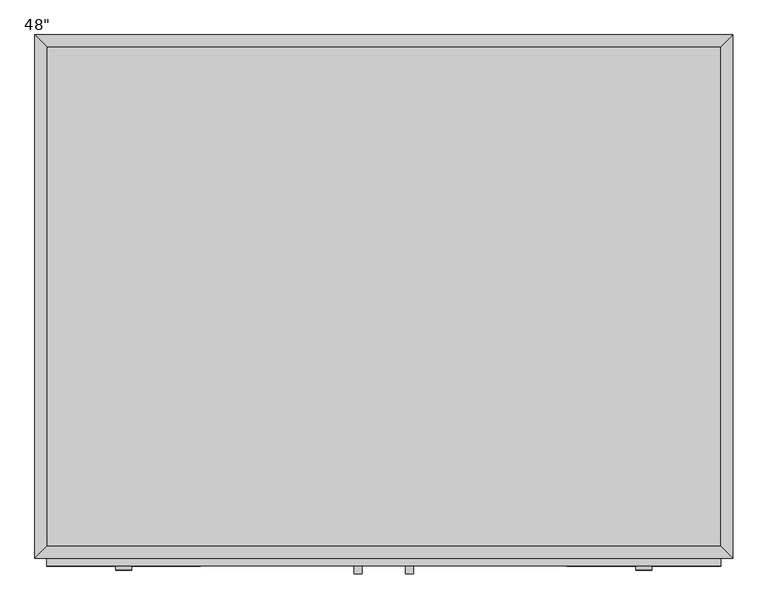
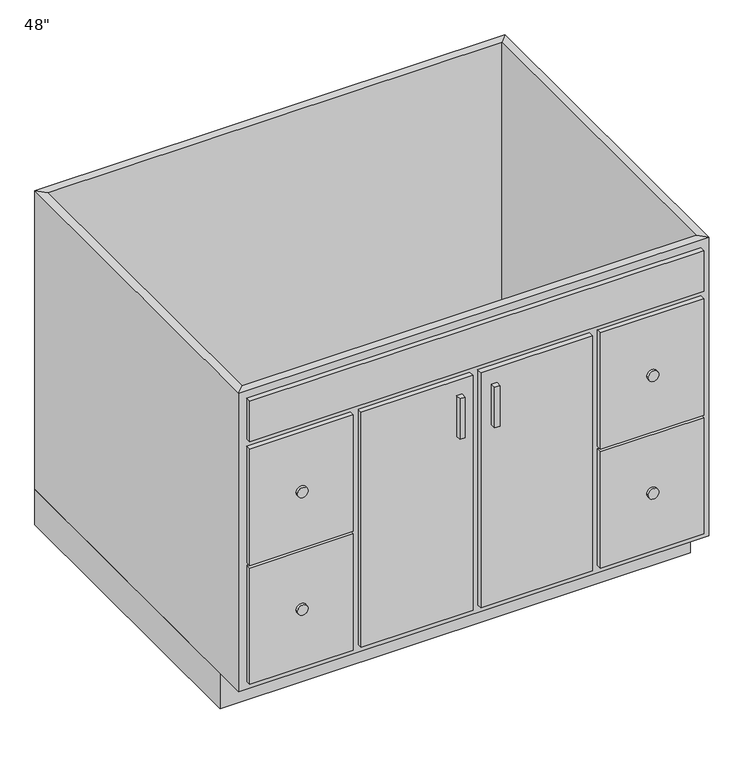
"""IFC4 building model written with IfcOpenShell, lengths in millimetres: furniture geometry."""

from ifc_helpers import new_model, si_unit, point, frame, frame_2d, origin, origin_with_axes, place, context, project, spatial, polyline, circle_curve, trimmed, segment, composite_curve, outline, extrude, faceted_brep, source, transform, mapped, element, save


def furniture_2d7fc6e7(model_context):
    return source(origin(), model_context, "Body", "SolidModel", [
        extrude(outline(polyline([(55.91996, -863.6), (43.21996, -863.6), (43.21996, -850.9), (55.91996, -850.9), (55.91996, -863.6)])), frame((0.0, 0.0, 558.8), z_axis=(0.0, 0.0, 1.0), x_axis=(1.0, 0.0, 0.0)), (0.0, 0.0, 1.0), 101.6),
        extrude(outline(polyline([(138.46996, -863.6), (125.76996, -863.6), (125.76996, -850.9), (138.46996, -850.9), (138.46996, -863.6)])), frame((0.0, 0.0, 558.8), z_axis=(0.0, 0.0, 1.0), x_axis=(1.0, 0.0, 0.0)), (0.0, 0.0, 1.0), 101.6),
        extrude(outline(composite_curve([segment(trimmed(circle_curve(frame_2d((550.8625, -325.87379)), 12.7), [point((550.8625, -338.57379))], [point((550.8625, -313.17379))], False, "CARTESIAN"), True, "CONTINUOUS"), segment(trimmed(circle_curve(frame_2d((550.8625, -325.87379)), 12.7), [point((550.8625, -313.17379))], [point((550.8625, -338.57379))], False, "CARTESIAN"), True, "CONTINUOUS")], self_intersect=False)), frame((0.0, -857.25, 0.0), z_axis=(0.0, 1.0, 0.0), x_axis=(0.0, 0.0, 1.0)), (0.0, 0.0, 1.0), 6.35),
        extrude(outline(composite_curve([segment(trimmed(circle_curve(frame_2d((255.5875, -325.87379)), 12.7), [point((255.5875, -338.57379))], [point((255.5875, -313.17379))], False, "CARTESIAN"), True, "CONTINUOUS"), segment(trimmed(circle_curve(frame_2d((255.5875, -325.87379)), 12.7), [point((255.5875, -313.17379))], [point((255.5875, -338.57379))], False, "CARTESIAN"), True, "CONTINUOUS")], self_intersect=False)), frame((0.0, -857.25, 0.0), z_axis=(0.0, 1.0, 0.0), x_axis=(0.0, 0.0, 1.0)), (0.0, 0.0, 1.0), 6.35),
        extrude(outline(composite_curve([segment(trimmed(circle_curve(frame_2d((255.5875, 507.56371)), 12.7), [point((255.5875, 494.86371))], [point((255.5875, 520.26371))], False, "CARTESIAN"), True, "CONTINUOUS"), segment(trimmed(circle_curve(frame_2d((255.5875, 507.56371)), 12.7), [point((255.5875, 520.26371))], [point((255.5875, 494.86371))], False, "CARTESIAN"), True, "CONTINUOUS")], self_intersect=False)), frame((0.0, -857.25, 0.0), z_axis=(0.0, 1.0, 0.0), x_axis=(0.0, 0.0, 1.0)), (0.0, 0.0, 1.0), 6.35),
        extrude(outline(composite_curve([segment(trimmed(circle_curve(frame_2d((550.8625, 507.56371)), 12.7), [point((550.8625, 494.86371))], [point((550.8625, 520.26371))], False, "CARTESIAN"), True, "CONTINUOUS"), segment(trimmed(circle_curve(frame_2d((550.8625, 507.56371)), 12.7), [point((550.8625, 520.26371))], [point((550.8625, 494.86371))], False, "CARTESIAN"), True, "CONTINUOUS")], self_intersect=False)), frame((0.0, -857.25, 0.0), z_axis=(0.0, 1.0, 0.0), x_axis=(0.0, 0.0, 1.0)), (0.0, 0.0, 1.0), 6.35),
        extrude(outline(polyline([(630.59496, -19.05), (630.59496, -819.15), (-448.90504, -819.15), (-448.90504, -19.05), (630.59496, -19.05)])), frame((0.0, 0.0, 88.9), z_axis=(0.0, 0.0, 1.0), x_axis=(1.0, 0.0, 0.0)), (0.0, 0.0, 1.0), 19.05),
        faceted_brep([(630.59496, -819.15, 838.2), (630.59496, -819.15, 88.9), (-448.90504, -819.15, 88.9), (-448.90504, -819.15, 838.2), (649.64496, -838.2, 838.2), (-467.95504, -838.2, 838.2), (649.64496, -838.2, 88.9), (-467.95504, -838.2, 88.9), (-448.90504, -19.05, 88.9), (-448.90504, -19.05, 838.2), (-467.95504, 0.0, 838.2), (-467.95504, 0.0, 88.9), (630.59496, -19.05, 88.9), (630.59496, -19.05, 838.2), (649.64496, 0.0, 838.2), (649.64496, 0.0, 88.9)], [[[0, 1, 2, 3]], [[4, 0, 3, 5]], [[6, 4, 5, 7]], [[1, 6, 7, 2]], [[3, 2, 8, 9]], [[5, 3, 9, 10]], [[7, 5, 10, 11]], [[2, 7, 11, 8]], [[9, 8, 12, 13]], [[10, 9, 13, 14]], [[11, 10, 14, 15]], [[8, 11, 15, 12]], [[13, 12, 1, 0]], [[14, 13, 0, 4]], [[15, 14, 4, 6]], [[12, 15, 6, 1]]]),
        extrude(outline(polyline([(649.64496, 0.0), (649.64496, -762.0), (-467.95504, -762.0), (-467.95504, 0.0), (649.64496, 0.0)])), origin_with_axes(), (0.0, 0.0, 1.0), 88.9),
        extrude(outline(polyline([(630.59496, -850.9), (-448.90504, -850.9), (-448.90504, -838.2), (630.59496, -838.2), (630.59496, -850.9)])), frame((0.0, 0.0, 717.55), z_axis=(0.0, 0.0, 1.0), x_axis=(1.0, 0.0, 0.0)), (0.0, 0.0, 1.0), 101.6),
        extrude(outline(polyline([(630.59496, -850.9), (384.53246, -850.9), (384.53246, -838.2), (630.59496, -838.2), (630.59496, -850.9)])), frame((0.0, 0.0, 406.4), z_axis=(0.0, 0.0, 1.0), x_axis=(1.0, 0.0, 0.0)), (0.0, 0.0, 1.0), 292.1),
        extrude(outline(polyline([(630.59496, -850.9), (384.53246, -850.9), (384.53246, -838.2), (630.59496, -838.2), (630.59496, -850.9)])), frame((0.0, 0.0, 107.95), z_axis=(0.0, 0.0, 1.0), x_axis=(1.0, 0.0, 0.0)), (0.0, 0.0, 1.0), 292.1),
        extrude(outline(polyline([(-202.84254, -850.9), (-448.90504, -850.9), (-448.90504, -838.2), (-202.84254, -838.2), (-202.84254, -850.9)])), frame((0.0, 0.0, 406.4), z_axis=(0.0, 0.0, 1.0), x_axis=(1.0, 0.0, 0.0)), (0.0, 0.0, 1.0), 292.1),
        extrude(outline(polyline([(-202.84254, -850.9), (-448.90504, -850.9), (-448.90504, -838.2), (-202.84254, -838.2), (-202.84254, -850.9)])), frame((0.0, 0.0, 107.95), z_axis=(0.0, 0.0, 1.0), x_axis=(1.0, 0.0, 0.0)), (0.0, 0.0, 1.0), 292.1),
        extrude(outline(polyline([(81.31996, -850.9), (-183.79254, -850.9), (-183.79254, -838.2), (81.31996, -838.2), (81.31996, -850.9)])), frame((0.0, 0.0, 107.95), z_axis=(0.0, 0.0, 1.0), x_axis=(1.0, 0.0, 0.0)), (0.0, 0.0, 1.0), 590.55),
        extrude(outline(polyline([(365.48246, -850.9), (100.36996, -850.9), (100.36996, -838.2), (365.48246, -838.2), (365.48246, -850.9)])), frame((0.0, 0.0, 107.95), z_axis=(0.0, 0.0, 1.0), x_axis=(1.0, 0.0, 0.0)), (0.0, 0.0, 1.0), 590.55),
    ])


if __name__ == "__main__":
    model = new_model("IFC4")
    model_context = context("Model", 3, world=origin())
    ifc_project = project(units=[si_unit("LENGTHUNIT", "METRE", prefix="MILLI")], contexts=[model_context])
    site = spatial("IfcSite", under=ifc_project)
    building = spatial("IfcBuilding", under=site)
    placement = place(None, origin())
    furniture_shape = furniture_2d7fc6e7(model_context)
    element("IfcFurniture", 1, ObjectType="48\"", at=placement, inside=building, context=model_context, shape_type="MappedRepresentation", body=[
        mapped(furniture_shape, transform((0.0, 0.0, 0.0), x_axis=(1.0, 0.0, 0.0), y_axis=(0.0, 1.0, 0.0), z_axis=(0.0, 0.0, 1.0))),
    ])
    save(model, "model.ifc")

# Revit data of these elements
# Type "48\""
#   Assembly Code = "C1030410"
#   Depth = 2' - 9"
#   Height = 2' - 9"
#   Toe Depth = 0' - 3"
#   Toe Height = 0' - 3 1/2"
#   Width = 3' - 8"
#   Cabinet Material = none
#   Door/Drawer Material = none
#   Handle Material = Cabinets - Handles
#   Default Elevation = 0
# Element 1 (IfcFurniture, "48\"")
#   Materials on its faces: "Cabinets", "Cabinets - Handles"
# Materials
#   "Cabinets - Handles": class "Metal", colour RGB 57 57 57, transparency 0
#   "Cabinets": colour RGB 249 249 249, transparency 0
